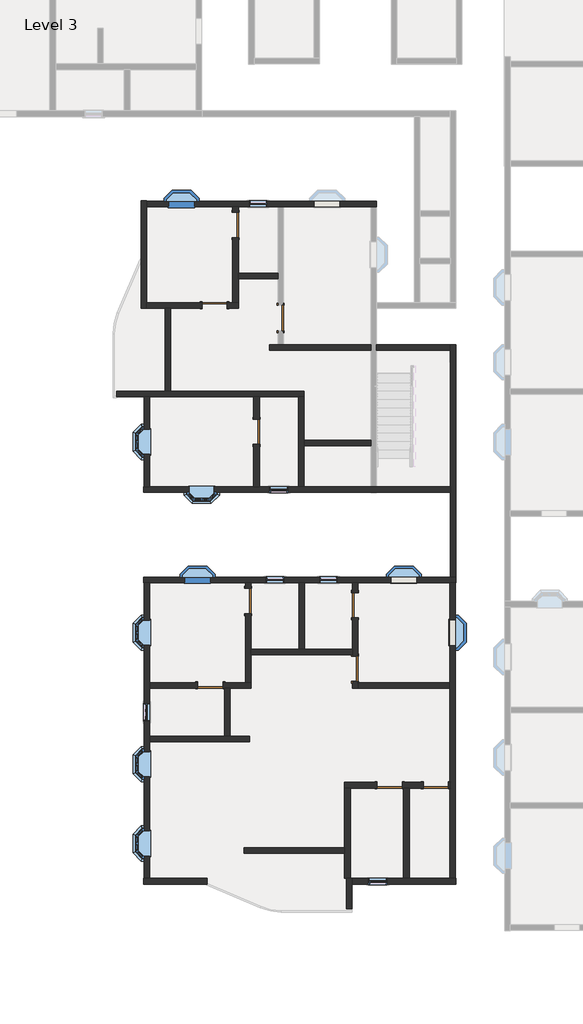
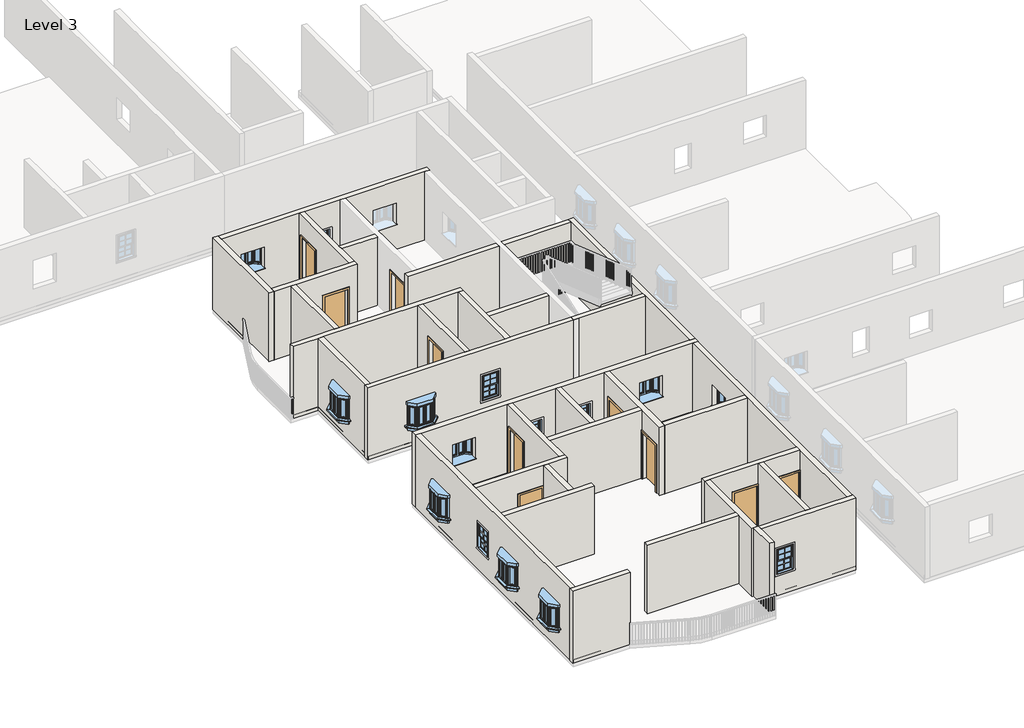
# One storey, part 1 of 14: 32 walls, 15 windows, 10 doors.
"""IFC4 building model written with IfcOpenShell, lengths in millimetres."""

from ifc_helpers import new_model, si_unit, frame, origin, place, context, project, spatial, polyline, outline, extrude, faceted_brep, transform, mapped, element, save
from components import door_54dd4da4, door_719f80de, window_910x910mm_67ef725a, window_8debb0fa

model = new_model("IFC4")

# Units and contexts
model_context = context("Model", 3, world=origin())
ifc_project = project(units=[si_unit("LENGTHUNIT", "METRE", prefix="MILLI")], contexts=[model_context])

# Site, building, storey
site = spatial("IfcSite", under=ifc_project)
building = spatial("IfcBuilding", under=site)
storey = spatial("IfcBuildingStorey", under=building, Name="Level 3", Elevation=6096.0)

# Doors
placement = place(None, origin())
door_shape = door_54dd4da4(model_context)
element("IfcDoor", 1, ObjectType="Single-Flush : 36\" x 84\"", at=placement, inside=storey, context=model_context, shape_type="MappedRepresentation", body=[
    mapped(door_shape, transform((-4626.037215, -17283.4916506, 6096.0), x_axis=(0.0, -1.0, 0.0), y_axis=(1.0, 0.0, 0.0), z_axis=(0.0, 0.0, 1.0))),
])
element("IfcDoor", 2, ObjectType="Single-Flush : 36\" x 84\"", at=placement, inside=storey, context=model_context, shape_type="MappedRepresentation", body=[
    mapped(door_shape, transform((-4626.037215, -14978.4416506, 6096.0), x_axis=(0.0, 1.0, 0.0), y_axis=(-1.0, 0.0, 0.0), z_axis=(0.0, 0.0, 1.0))),
])
element("IfcDoor", 3, ObjectType="Single-Flush : 36\" x 84\"", at=placement, inside=storey, context=model_context, shape_type="MappedRepresentation", body=[
    mapped(door_shape, transform((-9731.437215, -4100.8916506, 6096.0), x_axis=(1.0, 0.0, 0.0), y_axis=(0.0, 1.0, 0.0), z_axis=(0.0, 0.0, 1.0))),
])
element("IfcDoor", 4, ObjectType="Single-Flush : 36\" x 84\"", at=placement, inside=storey, context=model_context, shape_type="MappedRepresentation", body=[
    mapped(door_shape, transform((-7331.137215, -4558.0916506, 6096.0), x_axis=(0.0, -1.0, 0.0), y_axis=(1.0, 0.0, 0.0), z_axis=(0.0, 0.0, 1.0))),
])
door_2_shape = door_719f80de(model_context)
element("IfcDoor", 5, ObjectType="Single-Flush : 36\" x 84\"", at=placement, inside=storey, context=model_context, shape_type="MappedRepresentation", body=[
    mapped(door_2_shape, transform((-9883.837215, -17891.2072331, 6096.0), x_axis=(1.0, 0.0, 0.0), y_axis=(0.0, 1.0, 0.0), z_axis=(0.0, 0.0, 1.0))),
])
element("IfcDoor", 6, ObjectType="Single-Flush : 36\" x 84\"", at=placement, inside=storey, context=model_context, shape_type="MappedRepresentation", body=[
    mapped(door_2_shape, transform((-8512.237215, -14826.0416506, 6096.0), x_axis=(0.0, 1.0, 0.0), y_axis=(-1.0, 0.0, 0.0), z_axis=(0.0, 0.0, 1.0))),
])
element("IfcDoor", 7, ObjectType="Single-Flush : 36\" x 84\"", at=placement, inside=storey, context=model_context, shape_type="MappedRepresentation", body=[
    mapped(door_2_shape, transform((-8207.437215, -8691.9416506, 6096.0), x_axis=(0.0, 1.0, 0.0), y_axis=(-1.0, 0.0, 0.0), z_axis=(0.0, 0.0, 1.0))),
])
element("IfcDoor", 8, ObjectType="Single-Flush : 36\" x 84\"", at=placement, inside=storey, context=model_context, shape_type="MappedRepresentation", body=[
    mapped(door_2_shape, transform((-8969.437215, -1186.2416506, 6096.0), x_axis=(0.0, 1.0, 0.0), y_axis=(-1.0, 0.0, 0.0), z_axis=(0.0, 0.0, 1.0))),
])
element("IfcDoor", 9, ObjectType="Single-Flush : 36\" x 84\"", at=placement, inside=storey, context=model_context, shape_type="MappedRepresentation", body=[
    mapped(door_2_shape, transform((-3374.4891351, -21512.5916506, 6096.0), x_axis=(1.0, 0.0, 0.0), y_axis=(0.0, 1.0, 0.0), z_axis=(0.0, 0.0, 1.0))),
])
element("IfcDoor", 10, ObjectType="Single-Flush : 36\" x 84\"", at=placement, inside=storey, context=model_context, shape_type="MappedRepresentation", body=[
    mapped(door_2_shape, transform((-1698.0891351, -21512.5916506, 6096.0), x_axis=(1.0, 0.0, 0.0), y_axis=(0.0, 1.0, 0.0), z_axis=(0.0, 0.0, 1.0))),
])

# Walls
element("IfcWall", 11, ObjectType="4.5\" p", at=placement, inside=storey, context=model_context, shape_type="Brep", body=[
    faceted_brep([(-9426.637215, -17992.8072331, 8229.6), (-9426.637215, -17992.8072331, 6096.0), (-9375.837215, -17992.8072331, 6096.0), (-9172.637215, -17992.8072331, 6096.0), (-8410.637215, -17992.8072331, 6096.0), (-8410.637215, -17992.8072331, 9144.0), (-9172.637215, -17992.8072331, 9144.0), (-9375.837215, -17992.8072331, 9144.0), (-12087.287215, -17992.8072331, 9144.0), (-12087.287215, -17992.8072331, 6096.0), (-10341.037215, -17992.8072331, 6096.0), (-10341.037215, -17992.8072331, 8229.6), (-8410.637215, -17789.6072331, 6096.0), (-8613.837215, -17789.6072331, 6096.0), (-9426.637215, -17789.6072331, 6096.0), (-9426.637215, -17789.6072331, 8229.6), (-10341.037215, -17789.6072331, 8229.6), (-10341.037215, -17789.6072331, 6096.0), (-12087.287215, -17789.6072331, 6096.0), (-12087.287215, -17789.6072331, 9144.0), (-8613.837215, -17789.6072331, 9144.0), (-8410.637215, -17789.6072331, 9144.0)], [[[0, 1, 2, 3, 4, 5, 6, 7, 8, 9, 10, 11]], [[12, 13, 14, 15, 16, 17, 18, 19, 20, 21]], [[10, 9, 18, 17]], [[4, 3, 2, 1, 14, 13, 12]], [[8, 7, 6, 5, 21, 20, 19]], [[9, 8, 19, 18]], [[5, 4, 12, 21]], [[15, 14, 1, 0]], [[16, 15, 0, 11]], [[17, 16, 11, 10]]]),
])
element("IfcWall", 12, ObjectType="4.5\" p", at=placement, inside=storey, context=model_context, shape_type="Brep", body=[
    faceted_brep([(-8410.637215, -14368.8416506, 8229.6), (-8410.637215, -14368.8416506, 6096.0), (-8410.637215, -14165.6416506, 6096.0), (-8410.637215, -14165.6416506, 9144.0), (-8410.637215, -16572.2916506, 9144.0), (-8410.637215, -16775.4916506, 9144.0), (-8410.637215, -17789.6072331, 9144.0), (-8410.637215, -17789.6072331, 6096.0), (-8410.637215, -16775.4916506, 6096.0), (-8410.637215, -16572.2916506, 6096.0), (-8410.637215, -15283.2416506, 6096.0), (-8410.637215, -15283.2416506, 8229.6), (-8613.837215, -14165.6416506, 6096.0), (-8613.837215, -14368.8416506, 6096.0), (-8613.837215, -14368.8416506, 8229.6), (-8613.837215, -15283.2416506, 8229.6), (-8613.837215, -15283.2416506, 6096.0), (-8613.837215, -17789.6072331, 6096.0), (-8613.837215, -17789.6072331, 9144.0), (-8613.837215, -14165.6416506, 9144.0)], [[[0, 1, 2, 3, 4, 5, 6, 7, 8, 9, 10, 11]], [[12, 13, 14, 15, 16, 17, 18, 19]], [[2, 1, 13, 12]], [[10, 9, 8, 7, 17, 16]], [[6, 5, 4, 3, 19, 18]], [[7, 6, 18, 17]], [[3, 2, 12, 19]], [[14, 13, 1, 0]], [[15, 14, 0, 11]], [[16, 15, 11, 10]]]),
])
element("IfcWall", 13, ObjectType="4.5\" p", at=placement, inside=storey, context=model_context, shape_type="Brep", body=[
    faceted_brep([(-8410.637215, -16775.4916506, 6096.0), (-4727.637215, -16775.4916506, 6096.0), (-4727.637215, -16775.4916506, 9144.0), (-8410.637215, -16775.4916506, 9144.0), (-8410.637215, -16572.2916506, 6096.0), (-8410.637215, -16572.2916506, 9144.0), (-6670.737215, -16572.2916506, 9144.0), (-6467.537215, -16572.2916506, 9144.0), (-4727.637215, -16572.2916506, 9144.0), (-4727.637215, -16572.2916506, 6096.0), (-6467.537215, -16572.2916506, 6096.0), (-6670.737215, -16572.2916506, 6096.0)], [[[0, 1, 2, 3]], [[4, 5, 6, 7, 8, 9, 10, 11]], [[1, 0, 4, 11, 10, 9]], [[3, 2, 8, 7, 6, 5]], [[0, 3, 5, 4]], [[2, 1, 9, 8]]]),
])
element("IfcWall", 14, ObjectType="4.5\" p", at=placement, inside=storey, context=model_context, shape_type="SweptSolid", body=[
    extrude(outline(polyline([(-6670.737215, -16572.2916506), (-6670.737215, -14165.6416506), (-6467.537215, -14165.6416506), (-6467.537215, -16572.2916506), (-6670.737215, -16572.2916506)])), frame((0.0, 0.0, 6096.0), z_axis=(0.0, 0.0, 1.0), x_axis=(1.0, 0.0, 0.0)), (0.0, 0.0, 1.0), 3048.0),
])
element("IfcWall", 15, ObjectType="4.5\" p", at=placement, inside=storey, context=model_context, shape_type="Brep", body=[
    faceted_brep([(-4727.637215, -14165.6416506, 6096.0), (-4727.637215, -14521.2416506, 6096.0), (-4727.637215, -14521.2416506, 8229.6), (-4727.637215, -15435.6416506, 8229.6), (-4727.637215, -15435.6416506, 6096.0), (-4727.637215, -16572.2916506, 6096.0), (-4727.637215, -16775.4916506, 6096.0), (-4727.637215, -16826.2916506, 6096.0), (-4727.637215, -16826.2916506, 8229.6), (-4727.637215, -17740.6916506, 8229.6), (-4727.637215, -17740.6916506, 6096.0), (-4727.637215, -17994.6916506, 6096.0), (-4727.637215, -17994.6916506, 9144.0), (-4727.637215, -16775.4916506, 9144.0), (-4727.637215, -16572.2916506, 9144.0), (-4727.637215, -14165.6416506, 9144.0), (-4524.437215, -14521.2416506, 8229.6), (-4524.437215, -14521.2416506, 6096.0), (-4524.437215, -14165.6416506, 6096.0), (-4524.437215, -14165.6416506, 9144.0), (-4524.437215, -17791.4916506, 9144.0), (-4524.437215, -17994.6916506, 9144.0), (-4524.437215, -17994.6916506, 6096.0), (-4524.437215, -17791.4916506, 6096.0), (-4524.437215, -17740.6916506, 6096.0), (-4524.437215, -17740.6916506, 8229.6), (-4524.437215, -16826.2916506, 8229.6), (-4524.437215, -16826.2916506, 6096.0), (-4524.437215, -15435.6416506, 6096.0), (-4524.437215, -15435.6416506, 8229.6)], [[[0, 1, 2, 3, 4, 5, 6, 7, 8, 9, 10, 11, 12, 13, 14, 15]], [[16, 17, 18, 19, 20, 21, 22, 23, 24, 25, 26, 27, 28, 29]], [[11, 10, 24, 23, 22]], [[28, 27, 7, 6, 5, 4]], [[18, 17, 1, 0]], [[15, 14, 13, 12, 21, 20, 19]], [[0, 15, 19, 18]], [[12, 11, 22, 21]], [[25, 24, 10, 9]], [[26, 25, 9, 8]], [[27, 26, 8, 7]], [[2, 1, 17, 16]], [[3, 2, 16, 29]], [[4, 3, 29, 28]]]),
])
element("IfcWall", 16, ObjectType="4.5\" p", at=placement, inside=storey, context=model_context, shape_type="SweptSolid", body=[
    extrude(outline(polyline([(-4524.437215, -17791.4916506), (-1190.0891351, -17791.4916506), (-1190.0891351, -17994.6916506), (-4524.437215, -17994.6916506), (-4524.437215, -17791.4916506)])), frame((0.0, 0.0, 6096.0), z_axis=(0.0, 0.0, 1.0), x_axis=(1.0, 0.0, 0.0)), (0.0, 0.0, 1.0), 3048.0),
])
element("IfcWall", 17, ObjectType="4.5\" p", at=placement, inside=storey, context=model_context, shape_type="SweptSolid", body=[
    extrude(outline(polyline([(-9375.837215, -19734.5916506), (-9375.837215, -17992.8072331), (-9172.637215, -17992.8072331), (-9172.637215, -19734.5916506), (-9375.837215, -19734.5916506)])), frame((0.0, 0.0, 6096.0), z_axis=(0.0, 0.0, 1.0), x_axis=(1.0, 0.0, 0.0)), (0.0, 0.0, 1.0), 3048.0),
])
element("IfcWall", 18, ObjectType="4.5\" p", at=placement, inside=storey, context=model_context, shape_type="Brep", body=[
    faceted_brep([(-12087.287215, -19937.7916506, 6096.0), (-8455.087215, -19937.7916506, 6096.0), (-8455.087215, -19937.7916506, 9144.0), (-12087.287215, -19937.7916506, 9144.0), (-12087.287215, -19734.5916506, 6096.0), (-12087.287215, -19734.5916506, 9144.0), (-9375.837215, -19734.5916506, 9144.0), (-9172.637215, -19734.5916506, 9144.0), (-8455.087215, -19734.5916506, 9144.0), (-8455.087215, -19734.5916506, 6096.0), (-9172.637215, -19734.5916506, 6096.0), (-9375.837215, -19734.5916506, 6096.0)], [[[0, 1, 2, 3]], [[4, 5, 6, 7, 8, 9, 10, 11]], [[1, 0, 4, 11, 10, 9]], [[2, 1, 9, 8]], [[3, 2, 8, 7, 6, 5]], [[0, 3, 5, 4]]]),
])
element("IfcWall", 19, ObjectType="4.5\" p", at=placement, inside=storey, context=model_context, shape_type="Brep", body=[
    faceted_brep([(-13293.787215, -7421.9416506, 6096.0), (-12290.487215, -7421.9416506, 6096.0), (-12087.287215, -7421.9416506, 6096.0), (-8309.037215, -7421.9416506, 6096.0), (-8105.837215, -7421.9416506, 6096.0), (-6689.787215, -7421.9416506, 6096.0), (-6486.587215, -7421.9416506, 6096.0), (-6486.587215, -7421.9416506, 9144.0), (-6689.787215, -7421.9416506, 9144.0), (-8105.837215, -7421.9416506, 9144.0), (-8309.037215, -7421.9416506, 9144.0), (-12087.287215, -7421.9416506, 9144.0), (-12290.487215, -7421.9416506, 9144.0), (-13293.787215, -7421.9416506, 9144.0), (-13293.787215, -7218.7416506, 6096.0), (-13293.787215, -7218.7416506, 9144.0), (-11528.487215, -7218.7416506, 9144.0), (-11325.287215, -7218.7416506, 9144.0), (-6486.587215, -7218.7416506, 9144.0), (-6486.587215, -7218.7416506, 6096.0), (-11325.287215, -7218.7416506, 6096.0), (-11528.487215, -7218.7416506, 6096.0)], [[[0, 1, 2, 3, 4, 5, 6, 7, 8, 9, 10, 11, 12, 13]], [[14, 15, 16, 17, 18, 19, 20, 21]], [[6, 5, 4, 3, 2, 1, 0, 14, 21, 20, 19]], [[13, 12, 11, 10, 9, 8, 7, 18, 17, 16, 15]], [[0, 13, 15, 14]], [[7, 6, 19, 18]]]),
])
element("IfcWall", 20, ObjectType="4.5\" p", at=placement, inside=storey, context=model_context, shape_type="Brep", body=[
    faceted_brep([(-12201.587215, -4202.4916506, 6096.0), (-12201.587215, -3999.2916506, 6096.0), (-12201.587215, -525.8416506, 6096.0), (-12201.587215, -322.6416506, 6096.0), (-12201.587215, -309.9416506, 6096.0), (-12201.587215, -309.9416506, 9144.0), (-12201.587215, -322.6416506, 9144.0), (-12201.587215, -525.8416506, 9144.0), (-12201.587215, -3999.2916506, 9144.0), (-12201.587215, -4202.4916506, 9144.0), (-12404.787215, -4202.4916506, 6096.0), (-12404.787215, -4202.4916506, 9144.0), (-12404.787215, -309.9416506, 9144.0), (-12404.787215, -309.9416506, 6096.0)], [[[0, 1, 2, 3, 4, 5, 6, 7, 8, 9]], [[10, 11, 12, 13]], [[4, 3, 2, 1, 0, 10, 13]], [[5, 4, 13, 12]], [[9, 8, 7, 6, 5, 12, 11]], [[0, 9, 11, 10]]]),
])
element("IfcWall", 21, ObjectType="4.5\" p", at=placement, inside=storey, context=model_context, shape_type="Brep", body=[
    faceted_brep([(-9274.237215, -4202.4916506, 8229.6), (-9274.237215, -4202.4916506, 6096.0), (-8867.837215, -4202.4916506, 6096.0), (-8867.837215, -4202.4916506, 9144.0), (-11325.287215, -4202.4916506, 9144.0), (-11528.487215, -4202.4916506, 9144.0), (-12201.587215, -4202.4916506, 9144.0), (-12201.587215, -4202.4916506, 6096.0), (-11528.487215, -4202.4916506, 6096.0), (-11325.287215, -4202.4916506, 6096.0), (-10188.637215, -4202.4916506, 6096.0), (-10188.637215, -4202.4916506, 8229.6), (-8867.837215, -3999.2916506, 6096.0), (-9071.037215, -3999.2916506, 6096.0), (-9274.237215, -3999.2916506, 6096.0), (-9274.237215, -3999.2916506, 8229.6), (-10188.637215, -3999.2916506, 8229.6), (-10188.637215, -3999.2916506, 6096.0), (-12201.587215, -3999.2916506, 6096.0), (-12201.587215, -3999.2916506, 9144.0), (-9071.037215, -3999.2916506, 9144.0), (-8867.837215, -3999.2916506, 9144.0)], [[[0, 1, 2, 3, 4, 5, 6, 7, 8, 9, 10, 11]], [[12, 13, 14, 15, 16, 17, 18, 19, 20, 21]], [[2, 1, 14, 13, 12]], [[10, 9, 8, 7, 18, 17]], [[6, 5, 4, 3, 21, 20, 19]], [[7, 6, 19, 18]], [[3, 2, 12, 21]], [[15, 14, 1, 0]], [[16, 15, 0, 11]], [[17, 16, 11, 10]]]),
])
element("IfcWall", 22, ObjectType="4.5\" p", at=placement, inside=storey, context=model_context, shape_type="Brep", body=[
    faceted_brep([(-8867.837215, -729.0416506, 8229.6), (-8867.837215, -729.0416506, 6096.0), (-8867.837215, -525.8416506, 6096.0), (-8867.837215, -525.8416506, 9144.0), (-8867.837215, -2932.4916506, 9144.0), (-8867.837215, -3135.6916506, 9144.0), (-8867.837215, -3999.2916506, 9144.0), (-8867.837215, -3999.2916506, 6096.0), (-8867.837215, -3135.6916506, 6096.0), (-8867.837215, -2932.4916506, 6096.0), (-8867.837215, -1643.4416506, 6096.0), (-8867.837215, -1643.4416506, 8229.6), (-9071.037215, -525.8416506, 6096.0), (-9071.037215, -729.0416506, 6096.0), (-9071.037215, -729.0416506, 8229.6), (-9071.037215, -1643.4416506, 8229.6), (-9071.037215, -1643.4416506, 6096.0), (-9071.037215, -3999.2916506, 6096.0), (-9071.037215, -3999.2916506, 9144.0), (-9071.037215, -525.8416506, 9144.0)], [[[0, 1, 2, 3, 4, 5, 6, 7, 8, 9, 10, 11]], [[12, 13, 14, 15, 16, 17, 18, 19]], [[2, 1, 13, 12]], [[10, 9, 8, 7, 17, 16]], [[6, 5, 4, 3, 19, 18]], [[7, 6, 18, 17]], [[3, 2, 12, 19]], [[14, 13, 1, 0]], [[15, 14, 0, 11]], [[16, 15, 11, 10]]]),
])
element("IfcWall", 23, ObjectType="4.5\" p", at=placement, inside=storey, context=model_context, shape_type="SweptSolid", body=[
    extrude(outline(polyline([(-7432.737215, -3135.6916506), (-8867.837215, -3135.6916506), (-8867.837215, -2932.4916506), (-7432.737215, -2932.4916506), (-7432.737215, -3135.6916506)])), frame((0.0, 0.0, 6096.0), z_axis=(0.0, 0.0, 1.0), x_axis=(1.0, 0.0, 0.0)), (0.0, 0.0, 1.0), 3048.0),
])
element("IfcWall", 24, ObjectType="4.5\" p", at=placement, inside=storey, context=model_context, shape_type="Brep", body=[
    faceted_brep([(-7731.187215, -5726.4916506, 9144.0), (-7731.187215, -5726.4916506, 6096.0), (-4060.887215, -5726.4916506, 6096.0), (-4060.887215, -5726.4916506, 9144.0), (-7731.187215, -5523.2916506, 6096.0), (-7731.187215, -5523.2916506, 9144.0), (-7432.737215, -5523.2916506, 9144.0), (-7229.537215, -5523.2916506, 9144.0), (-4060.887215, -5523.2916506, 9144.0), (-4060.887215, -5523.2916506, 6096.0), (-7229.537215, -5523.2916506, 6096.0), (-7432.737215, -5523.2916506, 6096.0)], [[[0, 1, 2, 3]], [[4, 5, 6, 7, 8, 9, 10, 11]], [[1, 4, 11, 10, 9, 2]], [[5, 0, 3, 8, 7, 6]], [[1, 0, 5, 4]], [[3, 2, 9, 8]]]),
    faceted_brep([(-1177.3891351, -5726.4916506, 6096.0), (-1177.3891351, -5726.4916506, 9144.0), (-3857.687215, -5726.4916506, 9144.0), (-3857.687215, -5726.4916506, 6096.0), (-1177.3891351, -5523.2916506, 9144.0), (-1177.3891351, -5523.2916506, 6096.0), (-3857.687215, -5523.2916506, 6096.0), (-3857.687215, -5523.2916506, 9144.0)], [[[0, 1, 2, 3]], [[4, 5, 6, 7]], [[5, 0, 3, 6]], [[1, 4, 7, 2]], [[1, 0, 5, 4]], [[3, 2, 7, 6]]]),
])
element("IfcWall", 25, ObjectType="4.5\" p", at=placement, inside=storey, context=model_context, shape_type="SweptSolid", body=[
    extrude(outline(polyline([(-11528.487215, -7218.7416506), (-11528.487215, -4202.4916506), (-11325.287215, -4202.4916506), (-11325.287215, -7218.7416506), (-11528.487215, -7218.7416506)])), frame((0.0, 0.0, 6096.0), z_axis=(0.0, 0.0, 1.0), x_axis=(1.0, 0.0, 0.0)), (0.0, 0.0, 1.0), 3048.0),
])
element("IfcWall", 26, ObjectType="4.5\" p", at=placement, inside=storey, context=model_context, shape_type="SweptSolid", body=[
    extrude(outline(polyline([(-7421.9416506, 6096.0), (-8234.7416506, 6096.0), (-8234.7416506, 8229.6), (-9149.1416506, 8229.6), (-9149.1416506, 6096.0), (-10685.8416506, 6096.0), (-10685.8416506, 9144.0), (-7421.9416506, 9144.0), (-7421.9416506, 6096.0)])), frame((-8309.037215, 0.0, 0.0), z_axis=(1.0, 0.0, 0.0), x_axis=(0.0, 1.0, 0.0)), (0.0, 0.0, 1.0), 203.2),
])
element("IfcWall", 27, ObjectType="4.5\" p", at=placement, inside=storey, context=model_context, shape_type="Brep", body=[
    faceted_brep([(-6689.787215, -7421.9416506, 6096.0), (-6689.787215, -10685.8416506, 6096.0), (-6689.787215, -10685.8416506, 9144.0), (-6689.787215, -7421.9416506, 9144.0), (-6486.587215, -7421.9416506, 6096.0), (-6486.587215, -7421.9416506, 9144.0), (-6486.587215, -8990.3916506, 9144.0), (-6486.587215, -9193.5916506, 9144.0), (-6486.587215, -10685.8416506, 9144.0), (-6486.587215, -10685.8416506, 6096.0), (-6486.587215, -9193.5916506, 6096.0), (-6486.587215, -8990.3916506, 6096.0)], [[[0, 1, 2, 3]], [[4, 5, 6, 7, 8, 9, 10, 11]], [[1, 0, 4, 11, 10, 9]], [[3, 2, 8, 7, 6, 5]], [[0, 3, 5, 4]], [[2, 1, 9, 8]]]),
])
element("IfcWall", 28, ObjectType="4.5\" p", at=placement, inside=storey, context=model_context, shape_type="SweptSolid", body=[
    extrude(outline(polyline([(-4060.887215, -9193.5916506), (-6486.587215, -9193.5916506), (-6486.587215, -8990.3916506), (-4060.887215, -8990.3916506), (-4060.887215, -9193.5916506)])), frame((0.0, 0.0, 6096.0), z_axis=(0.0, 0.0, 1.0), x_axis=(1.0, 0.0, 0.0)), (0.0, 0.0, 1.0), 3048.0),
])
element("IfcWall", 29, ObjectType="9\"", at=placement, inside=storey, context=model_context, shape_type="Brep", body=[
    faceted_brep([(-1190.0891351, -21410.9916506, 6096.0), (-1240.8891351, -21410.9916506, 6096.0), (-1240.8891351, -21410.9916506, 8229.6), (-2155.2891351, -21410.9916506, 8229.6), (-2155.2891351, -21410.9916506, 6096.0), (-2917.2891351, -21410.9916506, 6096.0), (-2917.2891351, -21410.9916506, 8229.6), (-3831.6891351, -21410.9916506, 8229.6), (-3831.6891351, -21410.9916506, 6096.0), (-5006.4391351, -21410.9916506, 6096.0), (-5006.4391351, -21410.9916506, 9144.0), (-1190.0891351, -21410.9916506, 9144.0), (-1240.8891351, -21614.1916506, 8229.6), (-1240.8891351, -21614.1916506, 6096.0), (-1190.0891351, -21614.1916506, 6096.0), (-1190.0891351, -21614.1916506, 9144.0), (-2663.2891351, -21614.1916506, 9144.0), (-2866.4891351, -21614.1916506, 9144.0), (-4803.2391351, -21614.1916506, 9144.0), (-5006.4391351, -21614.1916506, 9144.0), (-5006.4391351, -21614.1916506, 6096.0), (-4803.2391351, -21614.1916506, 6096.0), (-3831.6891351, -21614.1916506, 6096.0), (-3831.6891351, -21614.1916506, 8229.6), (-2917.2891351, -21614.1916506, 8229.6), (-2917.2891351, -21614.1916506, 6096.0), (-2866.4891351, -21614.1916506, 6096.0), (-2663.2891351, -21614.1916506, 6096.0), (-2155.2891351, -21614.1916506, 6096.0), (-2155.2891351, -21614.1916506, 8229.6)], [[[0, 1, 2, 3, 4, 5, 6, 7, 8, 9, 10, 11]], [[12, 13, 14, 15, 16, 17, 18, 19, 20, 21, 22, 23, 24, 25, 26, 27, 28, 29]], [[22, 21, 20, 9, 8]], [[14, 13, 1, 0]], [[28, 27, 26, 25, 5, 4]], [[11, 10, 19, 18, 17, 16, 15]], [[0, 11, 15, 14]], [[10, 9, 20, 19]], [[6, 5, 25, 24]], [[7, 6, 24, 23]], [[8, 7, 23, 22]], [[2, 1, 13, 12]], [[3, 2, 12, 29]], [[4, 3, 29, 28]]]),
])
element("IfcWall", 30, ObjectType="9\"", at=placement, inside=storey, context=model_context, shape_type="Brep", body=[
    faceted_brep([(-5006.4391351, -21614.1916506, 6096.0), (-5006.4391351, -23779.5416506, 6096.0), (-5006.4391351, -23982.7416506, 6096.0), (-5006.4391351, -24897.1416506, 6096.0), (-5006.4391351, -24897.1416506, 9144.0), (-5006.4391351, -23982.7416506, 9144.0), (-5006.4391351, -23779.5416506, 9144.0), (-5006.4391351, -21614.1916506, 9144.0), (-4803.2391351, -21614.1916506, 6096.0), (-4803.2391351, -21614.1916506, 9144.0), (-4803.2391351, -24897.1416506, 9144.0), (-4803.2391351, -24897.1416506, 6096.0), (-4949.2891351, -24897.1416506, 6096.0), (-4949.2891351, -24897.1416506, 9144.0)], [[[0, 1, 2, 3, 4, 5, 6, 7]], [[8, 9, 10, 11]], [[3, 2, 1, 0, 8, 11, 12]], [[7, 6, 5, 4, 13, 10, 9]], [[0, 7, 9, 8]], [[4, 3, 12, 11, 10, 13]]]),
])
element("IfcWall", 31, ObjectType="9\"", at=placement, inside=storey, context=model_context, shape_type="SweptSolid", body=[
    extrude(outline(polyline([(-2866.4891351, -24897.1416506), (-2866.4891351, -21614.1916506), (-2663.2891351, -21614.1916506), (-2663.2891351, -24897.1416506), (-2866.4891351, -24897.1416506)])), frame((0.0, 0.0, 6096.0), z_axis=(0.0, 0.0, 1.0), x_axis=(1.0, 0.0, 0.0)), (0.0, 0.0, 1.0), 3048.0),
])
element("IfcWall", 32, ObjectType="9\"", at=placement, inside=storey, context=model_context, shape_type="SweptSolid", body=[
    extrude(outline(polyline([(-5006.4391351, -23982.7416506), (-8664.637215, -23982.7416506), (-8664.637215, -23779.5416506), (-5006.4391351, -23779.5416506), (-5006.4391351, -23982.7416506)])), frame((0.0, 0.0, 6096.0), z_axis=(0.0, 0.0, 1.0), x_axis=(1.0, 0.0, 0.0)), (0.0, 0.0, 1.0), 3048.0),
])
element("IfcWall", 33, ObjectType="9\" w", at=placement, inside=storey, context=model_context, shape_type="Brep", body=[
    faceted_brep([(-12303.187215, -14165.6416506, 6096.0), (-12290.487215, -14165.6416506, 6096.0), (-12087.287215, -14165.6416506, 6096.0), (-8613.837215, -14165.6416506, 6096.0), (-8410.637215, -14165.6416506, 6096.0), (-6670.737215, -14165.6416506, 6096.0), (-6467.537215, -14165.6416506, 6096.0), (-4727.637215, -14165.6416506, 6096.0), (-4524.437215, -14165.6416506, 6096.0), (-1190.0891351, -14165.6416506, 6096.0), (-986.8891351, -14165.6416506, 6096.0), (-961.4891351, -14165.6416506, 6096.0), (-961.4891351, -14165.6416506, 9144.0), (-986.8891351, -14165.6416506, 9144.0), (-1190.0891351, -14165.6416506, 9144.0), (-4524.437215, -14165.6416506, 9144.0), (-4727.637215, -14165.6416506, 9144.0), (-6467.537215, -14165.6416506, 9144.0), (-6670.737215, -14165.6416506, 9144.0), (-8410.637215, -14165.6416506, 9144.0), (-8613.837215, -14165.6416506, 9144.0), (-12087.287215, -14165.6416506, 9144.0), (-12290.487215, -14165.6416506, 9144.0), (-12303.187215, -14165.6416506, 9144.0), (-10805.562215, -14165.6416506, 8206.0), (-9895.562215, -14165.6416506, 8206.0), (-9895.562215, -14165.6416506, 7296.0), (-10805.562215, -14165.6416506, 7296.0), (-3312.2631751, -14165.6416506, 8206.0), (-2402.2631751, -14165.6416506, 8206.0), (-2402.2631751, -14165.6416506, 7296.0), (-3312.2631751, -14165.6416506, 7296.0), (-7870.887215, -14165.6416506, 8077.2), (-7210.487215, -14165.6416506, 8077.2), (-7210.487215, -14165.6416506, 7010.4), (-7870.887215, -14165.6416506, 7010.4), (-5927.787215, -14165.6416506, 8077.2), (-5267.387215, -14165.6416506, 8077.2), (-5267.387215, -14165.6416506, 7010.4), (-5927.787215, -14165.6416506, 7010.4), (-12303.187215, -13962.4416506, 6096.0), (-12303.187215, -13962.4416506, 9144.0), (-1177.3891351, -13962.4416506, 9144.0), (-974.1891351, -13962.4416506, 9144.0), (-961.4891351, -13962.4416506, 9144.0), (-961.4891351, -13962.4416506, 6096.0), (-974.1891351, -13962.4416506, 6096.0), (-1177.3891351, -13962.4416506, 6096.0), (-10805.562215, -13962.4416506, 8206.0), (-10805.562215, -13962.4416506, 7296.0), (-9895.562215, -13962.4416506, 7296.0), (-9895.562215, -13962.4416506, 8206.0), (-3312.2631751, -13962.4416506, 8206.0), (-3312.2631751, -13962.4416506, 7296.0), (-2402.2631751, -13962.4416506, 7296.0), (-2402.2631751, -13962.4416506, 8206.0), (-7870.887215, -13962.4416506, 8077.2), (-7870.887215, -13962.4416506, 7010.4), (-7210.487215, -13962.4416506, 7010.4), (-7210.487215, -13962.4416506, 8077.2), (-5927.787215, -13962.4416506, 8077.2), (-5927.787215, -13962.4416506, 7010.4), (-5267.387215, -13962.4416506, 7010.4), (-5267.387215, -13962.4416506, 8077.2)], [[[0, 1, 2, 3, 4, 5, 6, 7, 8, 9, 10, 11, 12, 13, 14, 15, 16, 17, 18, 19, 20, 21, 22, 23], [24, 25, 26, 27], [28, 29, 30, 31], [32, 33, 34, 35], [36, 37, 38, 39]], [[40, 41, 42, 43, 44, 45, 46, 47], [48, 49, 50, 51], [52, 53, 54, 55], [56, 57, 58, 59], [60, 61, 62, 63]], [[11, 10, 9, 8, 7, 6, 5, 4, 3, 2, 1, 0, 40, 47, 46, 45]], [[12, 11, 45, 44]], [[23, 22, 21, 20, 19, 18, 17, 16, 15, 14, 13, 12, 44, 43, 42, 41]], [[0, 23, 41, 40]], [[49, 48, 24, 27]], [[50, 49, 27, 26]], [[51, 50, 26, 25]], [[48, 51, 25, 24]], [[53, 52, 28, 31]], [[54, 53, 31, 30]], [[55, 54, 30, 29]], [[52, 55, 29, 28]], [[57, 56, 32, 35]], [[58, 57, 35, 34]], [[59, 58, 34, 33]], [[56, 59, 33, 32]], [[61, 60, 36, 39]], [[62, 61, 39, 38]], [[63, 62, 38, 37]], [[60, 63, 37, 36]]]),
])
element("IfcWall", 34, ObjectType="9\" w", at=placement, inside=storey, context=model_context, shape_type="Brep", body=[
    faceted_brep([(-10004.0323936, -24897.1416506, 6096.0), (-12087.287215, -24897.1416506, 6096.0), (-12290.487215, -24897.1416506, 6096.0), (-12303.187215, -24897.1416506, 6096.0), (-12303.187215, -24897.1416506, 9144.0), (-12290.487215, -24897.1416506, 9144.0), (-12087.287215, -24897.1416506, 9144.0), (-10004.0323936, -24897.1416506, 9144.0), (-10004.0323936, -25100.3416506, 6096.0), (-10004.0323936, -25100.3416506, 9144.0), (-12303.187215, -25100.3416506, 9144.0), (-12303.187215, -25100.3416506, 6096.0)], [[[0, 1, 2, 3, 4, 5, 6, 7]], [[8, 9, 10, 11]], [[3, 2, 1, 0, 8, 11]], [[4, 3, 11, 10]], [[7, 6, 5, 4, 10, 9]], [[0, 7, 9, 8]]]),
])
element("IfcWall", 35, ObjectType="9\" w", at=placement, inside=storey, context=model_context, shape_type="Brep", body=[
    faceted_brep([(-4746.0891351, -25989.3416506, 6096.0), (-4746.0891351, -25100.3416506, 6096.0), (-4746.0891351, -24897.1416506, 6096.0), (-4746.0891351, -24897.1416506, 9144.0), (-4746.0891351, -25100.3416506, 9144.0), (-4746.0891351, -25989.3416506, 9144.0), (-4949.2891351, -25989.3416506, 6096.0), (-4949.2891351, -25989.3416506, 9144.0), (-4949.2891351, -24897.1416506, 9144.0), (-4949.2891351, -24897.1416506, 6096.0), (-4803.2391351, -24897.1416506, 6096.0), (-4803.2391351, -24897.1416506, 9144.0)], [[[0, 1, 2, 3, 4, 5]], [[6, 7, 8, 9]], [[2, 1, 0, 6, 9, 10]], [[5, 4, 3, 11, 8, 7]], [[0, 5, 7, 6]], [[3, 2, 10, 9, 8, 11]]]),
])
element("IfcWall", 36, ObjectType="9\" w", at=placement, inside=storey, context=model_context, shape_type="Brep", body=[
    faceted_brep([(-4746.0891351, -25100.3416506, 6096.0), (-961.4891351, -25100.3416506, 6096.0), (-961.4891351, -25100.3416506, 9144.0), (-4746.0891351, -25100.3416506, 9144.0), (-3476.0891351, -25100.3416506, 8077.2), (-3476.0891351, -25100.3416506, 7010.4), (-4136.4891351, -25100.3416506, 7010.4), (-4136.4891351, -25100.3416506, 8077.2), (-4746.0891351, -24897.1416506, 6096.0), (-4746.0891351, -24897.1416506, 9144.0), (-2866.4891351, -24897.1416506, 9144.0), (-2663.2891351, -24897.1416506, 9144.0), (-1190.0891351, -24897.1416506, 9144.0), (-986.8891351, -24897.1416506, 9144.0), (-961.4891351, -24897.1416506, 9144.0), (-961.4891351, -24897.1416506, 6096.0), (-986.8891351, -24897.1416506, 6096.0), (-1190.0891351, -24897.1416506, 6096.0), (-2663.2891351, -24897.1416506, 6096.0), (-2866.4891351, -24897.1416506, 6096.0), (-3476.0891351, -24897.1416506, 8077.2), (-4136.4891351, -24897.1416506, 8077.2), (-4136.4891351, -24897.1416506, 7010.4), (-3476.0891351, -24897.1416506, 7010.4)], [[[0, 1, 2, 3], [4, 5, 6, 7]], [[8, 9, 10, 11, 12, 13, 14, 15, 16, 17, 18, 19], [20, 21, 22, 23]], [[1, 0, 8, 19, 18, 17, 16, 15]], [[2, 1, 15, 14]], [[3, 2, 14, 13, 12, 11, 10, 9]], [[0, 3, 9, 8]], [[5, 4, 20, 23]], [[6, 5, 23, 22]], [[7, 6, 22, 21]], [[4, 7, 21, 20]]]),
])
element("IfcWall", 37, ObjectType="9\" w", at=placement, inside=storey, context=model_context, shape_type="Brep", body=[
    faceted_brep([(-12290.487215, -14165.6416506, 6096.0), (-12290.487215, -24897.1416506, 6096.0), (-12290.487215, -24897.1416506, 9144.0), (-12290.487215, -14165.6416506, 9144.0), (-12290.487215, -16432.6244419, 7920.4), (-12290.487215, -16432.6244419, 7010.4), (-12290.487215, -15522.6244419, 7010.4), (-12290.487215, -15522.6244419, 7920.4), (-12290.487215, -21205.5916506, 7920.4), (-12290.487215, -21205.5916506, 7010.4), (-12290.487215, -20295.5916506, 7010.4), (-12290.487215, -20295.5916506, 7920.4), (-12290.487215, -24082.1416506, 7920.4), (-12290.487215, -24082.1416506, 7010.4), (-12290.487215, -23172.1416506, 7010.4), (-12290.487215, -23172.1416506, 7920.4), (-12290.487215, -19193.8994419, 8077.2), (-12290.487215, -19193.8994419, 7010.4), (-12290.487215, -18533.4994419, 7010.4), (-12290.487215, -18533.4994419, 8077.2), (-12087.287215, -14165.6416506, 6096.0), (-12087.287215, -14165.6416506, 9144.0), (-12087.287215, -17789.6072331, 9144.0), (-12087.287215, -17992.8072331, 9144.0), (-12087.287215, -19734.5916506, 9144.0), (-12087.287215, -19937.7916506, 9144.0), (-12087.287215, -24897.1416506, 9144.0), (-12087.287215, -24897.1416506, 6096.0), (-12087.287215, -19937.7916506, 6096.0), (-12087.287215, -19734.5916506, 6096.0), (-12087.287215, -17992.8072331, 6096.0), (-12087.287215, -17789.6072331, 6096.0), (-12087.287215, -16432.6244419, 7920.4), (-12087.287215, -15522.6244419, 7920.4), (-12087.287215, -15522.6244419, 7010.4), (-12087.287215, -16432.6244419, 7010.4), (-12087.287215, -21205.5916506, 7920.4), (-12087.287215, -20295.5916506, 7920.4), (-12087.287215, -20295.5916506, 7010.4), (-12087.287215, -21205.5916506, 7010.4), (-12087.287215, -24082.1416506, 7920.4), (-12087.287215, -23172.1416506, 7920.4), (-12087.287215, -23172.1416506, 7010.4), (-12087.287215, -24082.1416506, 7010.4), (-12087.287215, -19193.8994419, 8077.2), (-12087.287215, -18533.4994419, 8077.2), (-12087.287215, -18533.4994419, 7010.4), (-12087.287215, -19193.8994419, 7010.4)], [[[0, 1, 2, 3], [4, 5, 6, 7], [8, 9, 10, 11], [12, 13, 14, 15], [16, 17, 18, 19]], [[20, 21, 22, 23, 24, 25, 26, 27, 28, 29, 30, 31], [32, 33, 34, 35], [36, 37, 38, 39], [40, 41, 42, 43], [44, 45, 46, 47]], [[1, 0, 20, 31, 30, 29, 28, 27]], [[3, 2, 26, 25, 24, 23, 22, 21]], [[0, 3, 21, 20]], [[2, 1, 27, 26]], [[5, 4, 32, 35]], [[6, 5, 35, 34]], [[7, 6, 34, 33]], [[4, 7, 33, 32]], [[9, 8, 36, 39]], [[10, 9, 39, 38]], [[11, 10, 38, 37]], [[8, 11, 37, 36]], [[13, 12, 40, 43]], [[14, 13, 43, 42]], [[15, 14, 42, 41]], [[12, 15, 41, 40]], [[17, 16, 44, 47]], [[18, 17, 47, 46]], [[19, 18, 46, 45]], [[16, 19, 45, 44]]]),
])
element("IfcWall", 38, ObjectType="9\" w", at=placement, inside=storey, context=model_context, shape_type="Brep", body=[
    faceted_brep([(-1190.0891351, -14165.6416506, 6096.0), (-1190.0891351, -17791.4916506, 6096.0), (-1190.0891351, -17994.6916506, 6096.0), (-1190.0891351, -21410.9916506, 6096.0), (-1190.0891351, -21614.1916506, 6096.0), (-1190.0891351, -24897.1416506, 6096.0), (-1190.0891351, -24897.1416506, 9144.0), (-1190.0891351, -21614.1916506, 9144.0), (-1190.0891351, -21410.9916506, 9144.0), (-1190.0891351, -17994.6916506, 9144.0), (-1190.0891351, -17791.4916506, 9144.0), (-1190.0891351, -14165.6416506, 9144.0), (-1190.0891351, -15523.5666506, 8206.0), (-1190.0891351, -16433.5666506, 8206.0), (-1190.0891351, -16433.5666506, 7296.0), (-1190.0891351, -15523.5666506, 7296.0), (-986.8891351, -14165.6416506, 6096.0), (-986.8891351, -14165.6416506, 9144.0), (-986.8891351, -24897.1416506, 9144.0), (-986.8891351, -24897.1416506, 6096.0), (-986.8891351, -15523.5666506, 8206.0), (-986.8891351, -15523.5666506, 7296.0), (-986.8891351, -16433.5666506, 7296.0), (-986.8891351, -16433.5666506, 8206.0)], [[[0, 1, 2, 3, 4, 5, 6, 7, 8, 9, 10, 11], [12, 13, 14, 15]], [[16, 17, 18, 19], [20, 21, 22, 23]], [[5, 4, 3, 2, 1, 0, 16, 19]], [[11, 10, 9, 8, 7, 6, 18, 17]], [[0, 11, 17, 16]], [[6, 5, 19, 18]], [[21, 20, 12, 15]], [[22, 21, 15, 14]], [[23, 22, 14, 13]], [[20, 23, 13, 12]]]),
])
element("IfcWall", 39, ObjectType="9\" w", at=placement, inside=storey, context=model_context, shape_type="Brep", body=[
    faceted_brep([(-1177.3891351, -5523.2916506, 6096.0), (-1177.3891351, -5726.4916506, 6096.0), (-1177.3891351, -10685.8416506, 6096.0), (-1177.3891351, -10889.0416506, 6096.0), (-1177.3891351, -13962.4416506, 6096.0), (-1177.3891351, -13962.4416506, 9144.0), (-1177.3891351, -10889.0416506, 9144.0), (-1177.3891351, -10685.8416506, 9144.0), (-1177.3891351, -5726.4916506, 9144.0), (-1177.3891351, -5523.2916506, 9144.0), (-974.1891351, -5523.2916506, 6096.0), (-974.1891351, -5523.2916506, 9144.0), (-974.1891351, -13962.4416506, 9144.0), (-974.1891351, -13962.4416506, 6096.0)], [[[0, 1, 2, 3, 4, 5, 6, 7, 8, 9]], [[10, 11, 12, 13]], [[4, 3, 2, 1, 0, 10, 13]], [[9, 8, 7, 6, 5, 12, 11]], [[5, 4, 13, 12]], [[0, 9, 11, 10]]]),
])
element("IfcWall", 40, ObjectType="9\" w", at=placement, inside=storey, context=model_context, shape_type="Brep", body=[
    faceted_brep([(-1177.3891351, -10685.8416506, 6096.0), (-6486.587215, -10685.8416506, 6096.0), (-6689.787215, -10685.8416506, 6096.0), (-8105.837215, -10685.8416506, 6096.0), (-8309.037215, -10685.8416506, 6096.0), (-12087.287215, -10685.8416506, 6096.0), (-12290.487215, -10685.8416506, 6096.0), (-12303.187215, -10685.8416506, 6096.0), (-12303.187215, -10685.8416506, 9144.0), (-12290.487215, -10685.8416506, 9144.0), (-12087.287215, -10685.8416506, 9144.0), (-8309.037215, -10685.8416506, 9144.0), (-8105.837215, -10685.8416506, 9144.0), (-6689.787215, -10685.8416506, 9144.0), (-6486.587215, -10685.8416506, 9144.0), (-1177.3891351, -10685.8416506, 9144.0), (-9743.162215, -10685.8416506, 7920.4), (-10653.162215, -10685.8416506, 7920.4), (-10653.162215, -10685.8416506, 7010.4), (-9743.162215, -10685.8416506, 7010.4), (-7067.612215, -10685.8416506, 8077.2), (-7728.012215, -10685.8416506, 8077.2), (-7728.012215, -10685.8416506, 7010.4), (-7067.612215, -10685.8416506, 7010.4), (-1177.3891351, -10889.0416506, 6096.0), (-1177.3891351, -10889.0416506, 9144.0), (-12303.187215, -10889.0416506, 9144.0), (-12303.187215, -10889.0416506, 6096.0), (-9743.162215, -10889.0416506, 7920.4), (-9743.162215, -10889.0416506, 7010.4), (-10653.162215, -10889.0416506, 7010.4), (-10653.162215, -10889.0416506, 7920.4), (-7067.612215, -10889.0416506, 8077.2), (-7067.612215, -10889.0416506, 7010.4), (-7728.012215, -10889.0416506, 7010.4), (-7728.012215, -10889.0416506, 8077.2)], [[[0, 1, 2, 3, 4, 5, 6, 7, 8, 9, 10, 11, 12, 13, 14, 15], [16, 17, 18, 19], [20, 21, 22, 23]], [[24, 25, 26, 27], [28, 29, 30, 31], [32, 33, 34, 35]], [[7, 6, 5, 4, 3, 2, 1, 0, 24, 27]], [[8, 7, 27, 26]], [[15, 14, 13, 12, 11, 10, 9, 8, 26, 25]], [[0, 15, 25, 24]], [[29, 28, 16, 19]], [[30, 29, 19, 18]], [[31, 30, 18, 17]], [[28, 31, 17, 16]], [[33, 32, 20, 23]], [[34, 33, 23, 22]], [[35, 34, 22, 21]], [[32, 35, 21, 20]]]),
])
element("IfcWall", 41, ObjectType="9\" w", at=placement, inside=storey, context=model_context, shape_type="SweptSolid", body=[
    extrude(outline(polyline([(-10685.8416506, 6096.0), (-10685.8416506, 9144.0), (-7421.9416506, 9144.0), (-7421.9416506, 6096.0), (-10685.8416506, 6096.0)]), holes=[polyline([(-9508.8916506, 7920.4), (-9508.8916506, 7010.4), (-8598.8916506, 7010.4), (-8598.8916506, 7920.4), (-9508.8916506, 7920.4)])]), frame((-12290.487215, 0.0, 0.0), z_axis=(1.0, 0.0, 0.0), x_axis=(0.0, 1.0, 0.0)), (0.0, 0.0, 1.0), 203.2),
])
element("IfcWall", 42, ObjectType="9\" w", at=placement, inside=storey, context=model_context, shape_type="Brep", body=[
    faceted_brep([(-12201.587215, -525.8416506, 6096.0), (-9071.037215, -525.8416506, 6096.0), (-8867.837215, -525.8416506, 6096.0), (-7432.737215, -525.8416506, 6096.0), (-7229.537215, -525.8416506, 6096.0), (-4060.887215, -525.8416506, 6096.0), (-3857.687215, -525.8416506, 6096.0), (-3844.987215, -525.8416506, 6096.0), (-3844.987215, -525.8416506, 9144.0), (-3857.687215, -525.8416506, 9144.0), (-4060.887215, -525.8416506, 9144.0), (-7229.537215, -525.8416506, 9144.0), (-7432.737215, -525.8416506, 9144.0), (-8867.837215, -525.8416506, 9144.0), (-9071.037215, -525.8416506, 9144.0), (-12201.587215, -525.8416506, 9144.0), (-6100.212215, -525.8416506, 8206.0), (-5190.212215, -525.8416506, 8206.0), (-5190.212215, -525.8416506, 7296.0), (-6100.212215, -525.8416506, 7296.0), (-11386.587215, -525.8416506, 8206.0), (-10476.587215, -525.8416506, 8206.0), (-10476.587215, -525.8416506, 7296.0), (-11386.587215, -525.8416506, 7296.0), (-8480.487215, -525.8416506, 8077.2), (-7820.087215, -525.8416506, 8077.2), (-7820.087215, -525.8416506, 7010.4), (-8480.487215, -525.8416506, 7010.4), (-12201.587215, -322.6416506, 6096.0), (-12201.587215, -322.6416506, 9144.0), (-3844.987215, -322.6416506, 9144.0), (-3844.987215, -322.6416506, 6096.0), (-6100.212215, -322.6416506, 8206.0), (-6100.212215, -322.6416506, 7296.0), (-5190.212215, -322.6416506, 7296.0), (-5190.212215, -322.6416506, 8206.0), (-11386.587215, -322.6416506, 8206.0), (-11386.587215, -322.6416506, 7296.0), (-10476.587215, -322.6416506, 7296.0), (-10476.587215, -322.6416506, 8206.0), (-8480.487215, -322.6416506, 8077.2), (-8480.487215, -322.6416506, 7010.4), (-7820.087215, -322.6416506, 7010.4), (-7820.087215, -322.6416506, 8077.2)], [[[0, 1, 2, 3, 4, 5, 6, 7, 8, 9, 10, 11, 12, 13, 14, 15], [16, 17, 18, 19], [20, 21, 22, 23], [24, 25, 26, 27]], [[28, 29, 30, 31], [32, 33, 34, 35], [36, 37, 38, 39], [40, 41, 42, 43]], [[7, 6, 5, 4, 3, 2, 1, 0, 28, 31]], [[8, 7, 31, 30]], [[15, 14, 13, 12, 11, 10, 9, 8, 30, 29]], [[0, 15, 29, 28]], [[33, 32, 16, 19]], [[34, 33, 19, 18]], [[35, 34, 18, 17]], [[32, 35, 17, 16]], [[37, 36, 20, 23]], [[38, 37, 23, 22]], [[39, 38, 22, 21]], [[36, 39, 21, 20]], [[41, 40, 24, 27]], [[42, 41, 27, 26]], [[43, 42, 26, 25]], [[40, 43, 25, 24]]]),
])

# Windows
window_910x910mm_shape = window_910x910mm_67ef725a(model_context)
element("IfcWindow", 43, ObjectType="910x910mm", at=placement, inside=storey, context=model_context, shape_type="MappedRepresentation", body=[
    mapped(window_910x910mm_shape, transform((-10361.587215, -432.6982184, 6096.0), x_axis=(1.0, 0.0, 0.0), y_axis=(0.0, 1.0, 0.0), z_axis=(0.0, 0.0, 1.0))),
])
element("IfcWindow", 44, ObjectType="910x910mm", at=placement, inside=storey, context=model_context, shape_type="MappedRepresentation", body=[
    mapped(window_910x910mm_shape, transform((-12180.4306471, -8483.8916506, 5810.4), x_axis=(0.0, 1.0, 0.0), y_axis=(-1.0, 0.0, 0.0), z_axis=(0.0, 0.0, 1.0))),
])
element("IfcWindow", 45, ObjectType="910x910mm", at=placement, inside=storey, context=model_context, shape_type="MappedRepresentation", body=[
    mapped(window_910x910mm_shape, transform((-10768.162215, -10778.9850828, 5810.4), x_axis=(-1.0, 0.0, 0.0), y_axis=(0.0, -1.0, 0.0), z_axis=(0.0, 0.0, 1.0))),
])
element("IfcWindow", 46, ObjectType="910x910mm", at=placement, inside=storey, context=model_context, shape_type="MappedRepresentation", body=[
    mapped(window_910x910mm_shape, transform((-12180.4306471, -15407.6244419, 5810.4), x_axis=(0.0, 1.0, 0.0), y_axis=(-1.0, 0.0, 0.0), z_axis=(0.0, 0.0, 1.0))),
])
element("IfcWindow", 47, ObjectType="910x910mm", at=placement, inside=storey, context=model_context, shape_type="MappedRepresentation", body=[
    mapped(window_910x910mm_shape, transform((-9780.562215, -14072.4982184, 6096.0), x_axis=(1.0, 0.0, 0.0), y_axis=(0.0, 1.0, 0.0), z_axis=(0.0, 0.0, 1.0))),
])
element("IfcWindow", 48, ObjectType="910x910mm", at=placement, inside=storey, context=model_context, shape_type="MappedRepresentation", body=[
    mapped(window_910x910mm_shape, transform((-2287.2631751, -14072.4982184, 6096.0), x_axis=(1.0, 0.0, 0.0), y_axis=(0.0, 1.0, 0.0), z_axis=(0.0, 0.0, 1.0))),
])
element("IfcWindow", 49, ObjectType="910x910mm", at=placement, inside=storey, context=model_context, shape_type="MappedRepresentation", body=[
    mapped(window_910x910mm_shape, transform((-1096.945703, -16548.5666506, 6096.0), x_axis=(0.0, -1.0, 0.0), y_axis=(1.0, 0.0, 0.0), z_axis=(0.0, 0.0, 1.0))),
])
element("IfcWindow", 50, ObjectType="910x910mm", at=placement, inside=storey, context=model_context, shape_type="MappedRepresentation", body=[
    mapped(window_910x910mm_shape, transform((-12180.4306471, -20180.5916506, 5810.4), x_axis=(0.0, 1.0, 0.0), y_axis=(-1.0, 0.0, 0.0), z_axis=(0.0, 0.0, 1.0))),
])
element("IfcWindow", 51, ObjectType="910x910mm", at=placement, inside=storey, context=model_context, shape_type="MappedRepresentation", body=[
    mapped(window_910x910mm_shape, transform((-12180.4306471, -23057.1416506, 5810.4), x_axis=(0.0, 1.0, 0.0), y_axis=(-1.0, 0.0, 0.0), z_axis=(0.0, 0.0, 1.0))),
])
window_shape = window_8debb0fa(model_context)
element("IfcWindow", 52, ObjectType="Window-Double-Hung : 26\" x 42\"", at=placement, inside=storey, context=model_context, shape_type="MappedRepresentation", body=[
    mapped(window_shape, transform((-8150.287215, -424.2416506, 6096.0), x_axis=(1.0, 0.0, 0.0), y_axis=(0.0, 1.0, 0.0), z_axis=(0.0, 0.0, 1.0))),
])
element("IfcWindow", 53, ObjectType="Window-Double-Hung : 26\" x 42\"", at=placement, inside=storey, context=model_context, shape_type="MappedRepresentation", body=[
    mapped(window_shape, transform((-7397.812215, -10787.4416506, 6096.0), x_axis=(-1.0, 0.0, 0.0), y_axis=(0.0, -1.0, 0.0), z_axis=(0.0, 0.0, 1.0))),
])
element("IfcWindow", 54, ObjectType="Window-Double-Hung : 26\" x 42\"", at=placement, inside=storey, context=model_context, shape_type="MappedRepresentation", body=[
    mapped(window_shape, transform((-7540.687215, -14064.0416506, 6096.0), x_axis=(1.0, 0.0, 0.0), y_axis=(0.0, 1.0, 0.0), z_axis=(0.0, 0.0, 1.0))),
])
element("IfcWindow", 55, ObjectType="Window-Double-Hung : 26\" x 42\"", at=placement, inside=storey, context=model_context, shape_type="MappedRepresentation", body=[
    mapped(window_shape, transform((-5597.587215, -14064.0416506, 6096.0), x_axis=(1.0, 0.0, 0.0), y_axis=(0.0, 1.0, 0.0), z_axis=(0.0, 0.0, 1.0))),
])
element("IfcWindow", 56, ObjectType="Window-Double-Hung : 26\" x 42\"", at=placement, inside=storey, context=model_context, shape_type="MappedRepresentation", body=[
    mapped(window_shape, transform((-12188.887215, -18863.6994419, 6096.0), x_axis=(0.0, 1.0, 0.0), y_axis=(-1.0, 0.0, 0.0), z_axis=(0.0, 0.0, 1.0))),
])
element("IfcWindow", 57, ObjectType="Window-Double-Hung : 26\" x 42\"", at=placement, inside=storey, context=model_context, shape_type="MappedRepresentation", body=[
    mapped(window_shape, transform((-3806.2891351, -24998.7416506, 6096.0), x_axis=(-1.0, 0.0, 0.0), y_axis=(0.0, -1.0, 0.0), z_axis=(0.0, 0.0, 1.0))),
])

save(model, "model.ifc")

# Revit data of these elements
# Type "Single-Flush : 36\" x 84\""
#   Type Mark = "1"
#   Construction Type Id = "MDOOR"
#   Assembly Code = "C1020"
#   Analytic Construction = "Metal"
#   Thickness = 0' - 2"
#   Heat Transfer Coefficient (U) = 0.651978 BTU/(h·ft²·°F)
#   Height = 7' - 0"
#   Trim Projection Ext = 0' - 1"
#   Trim Projection Int = 0' - 1"
#   Trim Width = 0' - 3"
#   Width = 3' - 0"
#   Define Thermal Properties by = 1
#   Define Thermal Properties by = 1
#   Door Material = Door - Panel
#   Frame Material = Door - Frame
#   Visual Light Transmittance = 0
#   Solar Heat Gain Coefficient = 0
#   Function = (empty or 0)
#   Wall Closure = (empty or 0)
# Type "4.5\" p"
#   Assembly Code = "B2010"
#   Layers, outside or top first: 0' - 8" no material (function 1)
# Type "9\""
#   Assembly Code = "B2010"
#   Layers, outside or top first: 0' - 8" no material (function 1)
# Type "9\" w"
#   Assembly Code = "B2010"
#   Layers, outside or top first: 0' - 8" no material (function 1)
# Type "910x910mm"
#   Type Mark = "18"
#   Operation = "UserDefined"
#   Construction Type Id = "GSP4R"
#   Keynote = "L10"
#   Analytic Construction = "1/8 in Pilkington single glazing"
#   Wrap Layers (Ext) from Ext = 0' - 4.03543"
#   Wrap Layers (Int) from Ext = 0' - 6.98819"
#   Window Board Projection = 0' - 0.98425"
#   Window Board Extention = 0' - 0.98425"
#   Visual Light Transmittance = 0.9
#   Solar Heat Gain Coefficient = 0.78
#   Heat Transfer Coefficient (U) = 0.6496 BTU/(h·ft²·°F)
#   Glazing Thickness = 0' - 0.94488"
#   DONT CHANGE - Splay Width = 0' - 7.41997"
#   Rough Width = 2' - 11.82677"
#   Rough Height = 2' - 11.82677"
#   Roof Thickness = 0' - 4.92126"
#   Roof Overhang = 0' - 1.5748"
#   Plinth Thickness = 0' - 6.88976"
#   Height = 2' - 11.82677"
#   Width = 2' - 11.82677"
#   Frame Depth = 0' - 2.55906"
#   Default Head Height = 6' - 11.07087"
#   Cill Depth = 0' - 3.44488"
#   Cavity Closer Width = 0' - 1.9685"
#   Cavity Closer Offset from Ext = 0' - 4.03543"
#   Cavity Closer Depth = 0' - 3.34646"
#   Vis - Cavity Closers = yes
#   Define Thermal Properties by = 1
#   Material Trim = Window Frame
#   Material Glass = Glass
#   Material Frame = Window Frame
#   Manufacturer = ""
#   Wall Closure = (empty or 0)
# Type "Window-Double-Hung : 26\" x 42\""
#   Type Mark = "11"
#   Fire Rating = "0.5h"
#   Construction Type Id = "DG-DR"
#   Assembly Code = "B2020100"
#   Analytic Construction = "Double glazing - domestic"
#   Wall Thickness [instance default] = 0' - 6"
#   Window Inset [instance default] = 0' - 0"
#   Visual Light Transmittance = 0.81
#   Thermal Resistance (R) = 1.8146 (h·ft²·°F)/BTU
#   Solar Heat Gain Coefficient = 0.76
#   Muntin Width = 1' - 8"
#   Muntin Height = 1' - 5 1/8"
#   Interior Wall Closure [instance default] = 0' - 1 1/2"
#   Rough Width = 2' - 2 1/2"
#   Rough Height = 3' - 6 1/2"
#   Frame Extension [instance default] = 0' - 1 1/4"
#   Exterior Wall Closure [instance default] = 0' - 0 1/2"
#   Extension Jamb [instance default] = 0' - 1 1/2"
#   Heat Transfer Coefficient (U) = 0.5511 BTU/(h·ft²·°F)
#   Height = 3' - 6"
#   Width = 2' - 2"
#   Define Thermal Properties by = 1
#   Top Muntin Visibility = yes
#   Indicator Visibility [instance default] = yes
#   Extension Jamb Visibility [instance default] = yes
#   Interior Trim Visibility [instance default] = yes
#   Exterior Trim Visibility [instance default] = yes
#   Define Thermal Properties by = 1
#   Bottom Muntin Visibility = yes
#   Muntin Pattern = Muntin Pattern_2x2 : Muntin Pattern_2x2
#   Interior Trim Material = Wood - Stained
#   Interior Trim = Trim-Window-Interior-Flat : Picture Frame
#   Exterior Trim Material = Clad - White
#   Exterior Trim = Trim-Window-Exterior-Flat : with Sill
#   Glass Panel Material = Glass
#   Exterior Frame Material = Clad - White
#   Interior Frame Material = Wood - Stained
#   Wall Closure = (empty or 0)
# Elements 1, 2, 3, 4, 5, 6, 7, 8, 9, 10 (IfcDoor, "Single-Flush : 36\" x 84\"")
#   Phase Created = New Construction
#   Materials on its faces: "Door - Frame", "Door - Panel"
# Elements 11, 12, 13, 14, 15, 16, 17, 21, 22, 23, 24, 26, 27, 28 (IfcWall, "4.5\" p")
#   Top Offset = 0' - 0"
#   Base Offset = 0' - 0"
#   wall height = 10' - 0"
#   Phase Created = New Construction
#   Base Constraint = Level 3
#   Top Constraint = Level 4
#   Materials on its faces: "Default Wall"
# Element 18 (IfcWall, "4.5\" p")
#   Top Offset = 0' - 0"
#   Base Offset = 0' - 0"
#   wall height = 10' - 0"
#   Phase Created = New Construction
#   Base Constraint = Level 3
#   Top Constraint = Level 4
#   Materials on its faces: "Default Wall", "Door - Frame"
# Element 19 (IfcWall, "4.5\" p")
#   Top Offset = 0' - 0"
#   Base Offset = 0' - 0"
#   wall height = 10' - 0"
#   Phase Created = New Construction
#   Base Constraint = Level 3
#   Top Constraint = Level 4
#   Materials on its faces: "Default Wall", "Wood - Stained"
# Element 20 (IfcWall, "4.5\" p")
#   Top Offset = 0' - 0"
#   Base Offset = 0' - 0"
#   wall height = 10' - 0"
#   Phase Created = New Construction
#   Base Constraint = Level 3
#   Top Constraint = Level 4
#   Materials on its faces: "Default Wall", "Earth"
# Element 25 (IfcWall, "4.5\" p")
#   Top Offset = 0' - 0"
#   Base Offset = 0' - 0"
#   wall height = 10' - 0"
#   Phase Created = New Construction
#   Base Constraint = Level 3
#   Top Constraint = Level 4
#   Materials on its faces: "Default Wall", "Parking Stripe"
# Elements 29, 30, 31 (IfcWall, "9\"")
#   Top Offset = 0' - 0"
#   Base Offset = 0' - 0"
#   wall height = 10' - 0"
#   Phase Created = New Construction
#   Base Constraint = Level 3
#   Top Constraint = Level 4
#   Materials on its faces: "Default Wall"
# Element 32 (IfcWall, "9\"")
#   Top Offset = 0' - 0"
#   Base Offset = 0' - 0"
#   wall height = 10' - 0"
#   Phase Created = New Construction
#   Base Constraint = Level 3
#   Top Constraint = Level 4
#   Materials on its faces: "Default Wall", "Carpet (1)"
# Elements 33, 37 (IfcWall, "9\" w")
#   Top Offset = 0' - 0"
#   Base Offset = 0' - 0"
#   wall height = 10' - 0"
#   Phase Created = New Construction
#   Base Constraint = Level 3
#   Top Constraint = Level 4
#   Materials on its faces: "Default Wall", "Parking Stripe"
# Elements 34, 36 (IfcWall, "9\" w")
#   Top Offset = 0' - 0"
#   Base Offset = 0' - 0"
#   wall height = 10' - 0"
#   Phase Created = New Construction
#   Base Constraint = Level 3
#   Top Constraint = Level 4
#   Materials on its faces: "Default Wall", "Softwood, Lumber"
# Element 35 (IfcWall, "9\" w")
#   Top Offset = 0' - 0"
#   Base Offset = 0' - 0"
#   wall height = 10' - 0"
#   Phase Created = New Construction
#   Base Constraint = Level 3
#   Top Constraint = Level 4
#   Materials on its faces: "Default Wall", "Carpet (1)"
# Elements 38, 39, 42 (IfcWall, "9\" w")
#   Top Offset = 0' - 0"
#   Base Offset = 0' - 0"
#   wall height = 10' - 0"
#   Phase Created = New Construction
#   Base Constraint = Level 3
#   Top Constraint = Level 4
#   Materials on its faces: "Default Wall"
# Elements 40, 41 (IfcWall, "9\" w")
#   Top Offset = 0' - 0"
#   Base Offset = 0' - 0"
#   wall height = 10' - 0"
#   Phase Created = New Construction
#   Base Constraint = Level 3
#   Top Constraint = Level 4
#   Materials on its faces: "Default Wall", "Wood - Stained"
# Element 43 (IfcWindow, "910x910mm")
#   Mark = "123"
#   Phase Created = New Construction
#   Materials on its faces: "Window Frame", "Glass"
# Element 44 (IfcWindow, "910x910mm")
#   Mark = "125"
#   Phase Created = New Construction
#   Materials on its faces: "Window Frame", "Glass"
# Element 45 (IfcWindow, "910x910mm")
#   Mark = "126"
#   Phase Created = New Construction
#   Materials on its faces: "Window Frame", "Glass"
# Element 46 (IfcWindow, "910x910mm")
#   Mark = "127"
#   Phase Created = New Construction
#   Materials on its faces: "Window Frame", "Glass"
# Element 47 (IfcWindow, "910x910mm")
#   Mark = "128"
#   Phase Created = New Construction
#   Materials on its faces: "Window Frame", "Glass"
# Element 48 (IfcWindow, "910x910mm")
#   Mark = "129"
#   Phase Created = New Construction
#   Materials on its faces: "Window Frame", "Glass"
# Element 49 (IfcWindow, "910x910mm")
#   Mark = "130"
#   Phase Created = New Construction
#   Materials on its faces: "Window Frame", "Glass"
# Element 50 (IfcWindow, "910x910mm")
#   Mark = "131"
#   Phase Created = New Construction
#   Materials on its faces: "Window Frame", "Glass"
# Element 51 (IfcWindow, "910x910mm")
#   Mark = "132"
#   Phase Created = New Construction
#   Materials on its faces: "Window Frame", "Glass"
# Element 52 (IfcWindow, "Window-Double-Hung : 26\" x 42\"")
#   Mark = "158"
#   Window Inset = 0' - 0"
#   Interior Wall Closure = 0' - 1 1/2"
#   Frame Extension = 0' - 1 1/4"
#   Exterior Wall Closure = 0' - 0 1/2"
#   Interior Trim Visibility = yes
#   Indicator Visibility = yes
#   Exterior Trim Visibility = yes
#   Phase Created = New Construction
#   Materials on its faces: "Wood - Stained", "Glass", "Clad - White"
# Element 53 (IfcWindow, "Window-Double-Hung : 26\" x 42\"")
#   Mark = "159"
#   Window Inset = 0' - 0"
#   Interior Wall Closure = 0' - 1 1/2"
#   Frame Extension = 0' - 1 1/4"
#   Exterior Wall Closure = 0' - 0 1/2"
#   Interior Trim Visibility = yes
#   Indicator Visibility = yes
#   Exterior Trim Visibility = yes
#   Phase Created = New Construction
#   Materials on its faces: "Wood - Stained", "Glass", "Clad - White"
# Element 54 (IfcWindow, "Window-Double-Hung : 26\" x 42\"")
#   Mark = "160"
